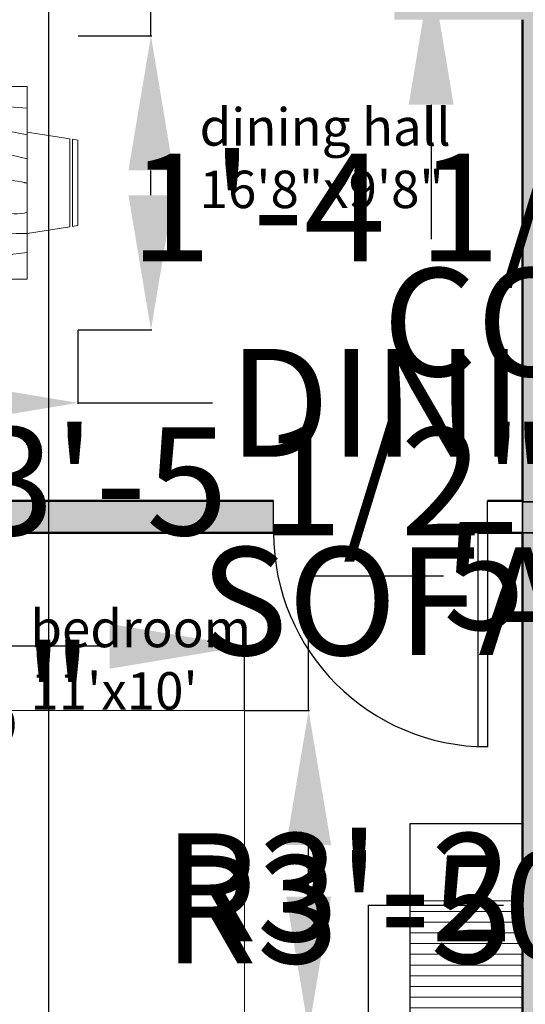
# Model space of a CAD drawing. Units: inches. Extents: x 25 to 82118, y 10 to 6494.
# Tile 4 of 9: x 40833 to 40928, y 3189 to 3373. Entities that reach past the tile are written whole.
import ezdxf

# ---------------------------------------------------------------- set-up
doc = ezdxf.new("R2010")
doc.units = ezdxf.units.IN
doc.header["$MEASUREMENT"] = 0
for name, color, linetype, lineweight in [('A-ANNO-DIMS', 2, 'Continuous', 18), ('A-AREA-IDEN', 7, 'Continuous', 25), ('A-DOOR', 3, 'Continuous', 25), ('A-FLOR-CASE', 8, 'Continuous', 25), ('A-FLOR-CASE-PATT', 9, 'Continuous', 13), ('A-FURN', 8, 'Continuous', 18), ('A-WALL', 7, 'Continuous', 50)]:
    doc.layers.add(name, color=color, linetype=linetype, lineweight=lineweight)
doc.layers.add('A-COLS', color=30, linetype='Continuous', lineweight=35, true_color=0xf26722)
doc.layers.add('A-WALL-PATT', color=18, linetype='Continuous', lineweight=13, true_color=0x000000)
doc.styles.get("Standard").update_dxf_attribs({"font": 'arial.ttf'})
doc.dimstyles.get("Standard").update_dxf_attribs({"dimtxt": 20.18, "dimasz": 25.18, "dimexe": 0.18, "dimexo": 0.0625, "dimgap": 0.09, "dimtad": 0, "dimtih": 1, "dimtoh": 1, "dimdec": 0, "dimzin": 0, "dimdsep": 46, "dimlunit": 3, "dimtxsty": 'Standard', "dimcen": 0.09, "dimadec": 0, "dimazin": 0, "dimtfac": 1, "dimtdec": 0, "dimtofl": 0, "dimtmove": 0, "dimatfit": 3, "dimfxl": 1, "dimtolj": 1, "dimtzin": 0, "dimarcsym": 0})

# ---------------------------------------------------------------- blocks, each defined once
blk = doc.blocks.new('Bed - Queen')
for p, q in [((0, -80.00003), (0, 0)), ((0, 0), (59.99999, 0)), ((59.99999, 0), (59.99999, -80.00003)), ((7.99999, -1.2), (28.79998, -1.2)), ((7.99999, -14.4), (7.99999, -1.2)), ((28.79998, -1.2), (28.79998, -14.4)), ((31.19999, -1.2), (51.99999, -1.2)), ((31.19999, -14.4), (31.19999, -1.2)), ((51.99999, -1.2), (51.99999, -16.4)), ((0, -14.4), (44.8, -14.4)), ((59.99999, -29.6), (44.8, -14.4)), ((44.8, -14.4), (44.8, -29.6)), ((51.99999, -16.4), (46.79936, -16.4)), ((44.8, -16.8), (0, -16.8)), ((44.8, -29.6), (59.99999, -29.6)), ((59.99999, -80.00003), (0, -80.00003))]:
    blk.add_line(p, q)
blk = doc.blocks.new('Dining Set - 36 x 72 in.')
for p, q in [((-22.2343, 26.00059), (-23.4847, 17.99762)), ((-22.2304, 26), (-5.7608, 26)), ((-22, 27.5), (-22.1562, 26.50042)), ((-5.8416, 26.5), (-22.1534, 26.5)), ((-22, 27.5), (-6, 27.5)), ((-5.8437, 26.49966), (-6, 27.5)), ((-4.5152, 17.99762), (-5.7655, 25.99926)), ((5.7657, 26.00059), (4.5153, 17.99762)), ((5.7696, 26), (22.2392, 26)), ((6, 27.5), (5.8438, 26.50042)), ((22.1584, 26.5), (5.8466, 26.5)), ((6, 27.5), (22, 27.5)), ((22.1563, 26.49966), (22, 27.5)), ((23.4848, 17.99762), (22.2345, 25.99926)), ((36, 18), (-36, 18)), ((-36, 18), (-36, -18)), ((36, -18), (36, 18)), ((-44.0006, 8.23428), (-35.9976, 9.48474)), ((44.0006, 8.23428), (35.9976, 9.48474)), ((-45.5, 8), (-44.5004, 8.15617)), ((-45.5, 8), (-45.5, -8)), ((-44.5, -8.15843), (-44.5, 8.15338)), ((-44, 8.23041), (-44, -8.23915)), ((44, 8.23041), (44, -8.23915)), ((44.5, -8.15843), (44.5, 8.15338)), ((45.5, 8), (44.5005, 8.15617)), ((45.5, 8), (45.5, -8)), ((-44.4997, -8.15631), (-45.5, -8)), ((-35.9976, -9.48476), (-43.9993, -8.2345)), ((35.9976, -9.48476), (43.9993, -8.2345)), ((44.4997, -8.15631), (45.5, -8)), ((-36, -18), (36, -18)), ((-22.2343, -26.0006), (-23.4847, -17.99762)), ((-4.5152, -17.99762), (-5.7655, -25.99928)), ((5.7657, -26.0006), (4.5153, -17.99762)), ((23.4848, -17.99762), (22.2345, -25.99928)), ((-22.2304, -26), (-5.7608, -26)), ((-22, -27.5), (-22.1562, -26.50044)), ((-5.8416, -26.5), (-22.1534, -26.5)), ((-22, -27.5), (-6, -27.5)), ((-5.8437, -26.49967), (-6, -27.5)), ((5.7696, -26), (22.2392, -26)), ((6, -27.5), (5.8438, -26.50044)), ((22.1584, -26.5), (5.8466, -26.5)), ((6, -27.5), (22, -27.5)), ((22.1563, -26.49967), (22, -27.5))]:
    blk.add_line(p, q)
for points in [[(-36, 15), (-31.1772, 14.97754), (-26.8079, 14.91406), (-22.8538, 14.81543), (-19.276, 14.6875), (-16.0362, 14.53613), (-13.0957, 14.36718), (-10.4159, 14.18652), (-7.9583, 14), (-5.6904, 13.81315), (-3.6035, 13.63021), (-1.6954, 13.45508), (0.0365, 13.29166), (1.5945, 13.14388), (2.9811, 13.01562), (4.1988, 12.9108), (5.25, 12.83333), (6.1393, 12.78613), (6.8802, 12.76823), (7.4883, 12.77767), (7.9792, 12.8125), (8.3685, 12.87077), (8.6719, 12.95052), (8.9049, 13.0498), (9.0833, 13.16666), (9.2205, 13.29899), (9.3216, 13.44401), (9.3895, 13.59879), (9.4271, 13.76041), (9.4373, 13.92594), (9.4232, 14.09245), (9.3875, 14.257), (9.3333, 14.41666), (9.2638, 14.56917), (9.1836, 14.71484), (9.0975, 14.85465), (9.0104, 14.98958), (8.9272, 15.1206), (8.8529, 15.2487), (8.7922, 15.37483), (8.75, 15.5), (8.7305, 15.62467), (8.7344, 15.74739), (8.7617, 15.86621), (8.8125, 15.97916), (8.8867, 16.08431), (8.9844, 16.17968), (9.1055, 16.26334), (9.25, 16.33333), (9.4189, 16.38802), (9.6172, 16.42708), (9.8506, 16.45052), (10.125, 16.45833), (10.4463, 16.45052), (10.8203, 16.42708), (11.2529, 16.38802), (11.75, 16.33333), (12.3184, 16.26318), (12.9694, 16.17838), (13.7151, 16.07991), (14.5677, 15.96875), (15.5395, 15.84586), (16.6426, 15.71224), (17.8893, 15.56884), (19.2917, 15.41666), (20.859, 15.25667), (22.5879, 15.08984), (24.4721, 14.91715), (26.5052, 14.73958), (28.6809, 14.5581), (30.9929, 14.3737), (33.4347, 14.18733), (36, 14)], [(-36, 10), (-28.9766, 10.14274), (-23.1725, 10.20442), (-18.4241, 10.19775), (-14.5677, 10.13541), (-11.4399, 10.03011), (-8.877, 9.89453), (-6.7154, 9.74137), (-4.7917, 9.58333), (-2.9698, 9.43082), (-1.2246, 9.28515), (0.4415, 9.14534), (2.026, 9.01041), (3.5266, 8.87939), (4.9408, 8.7513), (6.266, 8.62516), (7.5, 8.5), (8.6411, 8.37549), (9.6914, 8.2539), (10.6538, 8.13818), (11.5312, 8.03125), (12.3267, 7.93603), (13.043, 7.85547), (13.6831, 7.79248), (14.25, 7.75), (14.7471, 7.7303), (15.1797, 7.73307), (15.5537, 7.75732), (15.875, 7.80208), (16.1494, 7.86637), (16.3828, 7.94922), (16.5811, 8.04964), (16.75, 8.16666), (16.8944, 8.29915), (17.0143, 8.44531), (17.1089, 8.60319), (17.1771, 8.77083), (17.218, 8.94629), (17.2305, 9.1276), (17.2137, 9.31282), (17.1667, 9.5), (17.0895, 9.6875), (16.987, 9.875), (16.8649, 10.0625), (16.7292, 10.25), (16.5856, 10.4375), (16.4401, 10.625), (16.2985, 10.8125), (16.1667, 11), (16.05, 11.18733), (15.9518, 11.3737), (15.8752, 11.5581), (15.8229, 11.73958), (15.798, 11.91715), (15.8034, 12.08984), (15.842, 12.25667), (15.9167, 12.41666), (16.0295, 12.56836), (16.1784, 12.70833), (16.3605, 12.83268), (16.5729, 12.9375), (16.8127, 13.01888), (17.0768, 13.07291), (17.3625, 13.0957), (17.6667, 13.08333), (17.9894, 13.03312), (18.3418, 12.94726), (18.7382, 12.82918), (19.1927, 12.68229), (19.7195, 12.51001), (20.3327, 12.31575), (21.0465, 12.10294), (21.875, 11.875), (22.8357, 11.63354), (23.959, 11.37304), (25.2786, 11.08618), (26.8282, 10.76562), (28.6414, 10.40405), (30.752, 9.99414), (33.1936, 9.52856), (36, 9)], [(-36, 5.5), (-30.7157, 5.3348), (-26.069, 5.20963), (-21.9946, 5.11767), (-18.4271, 5.05208), (-15.3009, 5.00602), (-12.5508, 4.97265), (-10.1112, 4.94515), (-7.9167, 4.91666), (-5.909, 4.88167), (-4.0586, 4.83984), (-2.3429, 4.79215), (-0.7396, 4.73958), (0.7739, 4.6831), (2.22, 4.6237), (3.6213, 4.56233), (5, 4.5), (6.373, 4.43782), (7.7344, 4.3776), (9.0723, 4.32129), (10.375, 4.27083), (11.6309, 4.22819), (12.8281, 4.19531), (13.9551, 4.17415), (15, 4.16666), (15.954, 4.17448), (16.819, 4.19791), (17.6001, 4.23698), (18.3021, 4.29166), (18.9299, 4.36198), (19.4883, 4.44791), (19.9823, 4.54948), (20.4167, 4.66666), (20.7969, 4.79899), (21.1302, 4.94401), (21.4245, 5.09879), (21.6875, 5.26041), (21.9271, 5.42594), (22.1511, 5.59245), (22.3672, 5.757), (22.5834, 5.91666), (22.8065, 6.06868), (23.0404, 6.21093), (23.2879, 6.34147), (23.5521, 6.45833), (23.8358, 6.55957), (24.142, 6.64323), (24.4735, 6.70735), (24.8334, 6.75), (25.2235, 6.76969), (25.642, 6.76692), (26.0858, 6.74267), (26.5521, 6.69791), (27.0379, 6.63362), (27.5404, 6.55078), (28.0565, 6.45036), (28.5834, 6.33333), (29.1242, 6.19987), (29.7071, 6.04687), (30.3661, 5.87044), (31.1354, 5.66666), (32.0493, 5.43164), (33.142, 5.16146), (34.4475, 4.85221), (36, 4.5)], [(-36, -1), (-30.7915, -0.6591), (-26.0195, -0.38216), (-21.6519, -0.16284), (-17.6563, 0.00521), (-14.0005, 0.12833), (-10.6523, 0.21289), (-7.5796, 0.26522), (-4.75, 0.29166), (-2.134, 0.29793), (0.2878, 0.28711), (2.5317, 0.26163), (4.6146, 0.22396), (6.5529, 0.17651), (8.3633, 0.12174), (10.0623, 0.06209), (11.6667, 0), (13.1899, -0.06201), (14.6341, -0.1211), (15.9982, -0.17432), (17.2813, -0.21875), (18.4823, -0.25147), (19.6003, -0.26953), (20.6343, -0.27002), (21.5834, -0.25), (22.4481, -0.20768), (23.2357, -0.14584), (23.9549, -0.06836), (24.6146, 0.02083), (25.2235, 0.11784), (25.7904, 0.21875), (26.3241, 0.31966), (26.8334, 0.41666), (27.3265, 0.50618), (27.8099, 0.58593), (28.2894, 0.65397), (28.7709, 0.70833), (29.2601, 0.74707), (29.763, 0.76823), (30.2855, 0.76985), (30.8334, 0.75), (31.4088, 0.70784), (31.9994, 0.64713), (32.589, 0.57275), (33.1615, 0.48958), (33.7008, 0.4025), (34.1908, 0.3164), (34.6153, 0.23616), (34.9584, 0.16666), (35.2099, 0.11165), (35.3848, 0.07031), (35.504, 0.04069), (35.5886, 0.02083), (35.6594, 0.00879), (35.7377, 0.0026), (35.8442, 0.00032), (36, 0)], [(-36, -6.5), (-27.1843, -6.31267), (-20.084, -6.1263), (-14.469, -5.9419), (-10.1094, -5.76042), (-6.7752, -5.58285), (-4.2363, -5.41016), (-2.2629, -5.24333), (-0.625, -5.08334), (0.8708, -4.93099), (2.2715, -4.78646), (3.5872, -4.64974), (4.8281, -4.52084), (6.0046, -4.39974), (7.127, -4.28646), (8.2053, -4.18099), (9.25, -4.08334), (10.2705, -3.99382), (11.2734, -3.91407), (12.2647, -3.84603), (13.25, -3.79167), (14.2354, -3.75293), (15.2266, -3.73177), (16.2295, -3.73015), (17.25, -3.75), (18.2912, -3.79248), (19.3451, -3.85547), (20.4009, -3.93604), (21.4479, -4.03125), (22.4754, -4.13819), (23.4727, -4.25391), (24.4289, -4.37549), (25.3334, -4.5), (26.1785, -4.62492), (26.9694, -4.74935), (27.7145, -4.87281), (28.4219, -4.99479), (29.1, -5.11483), (29.7572, -5.23242), (30.4016, -5.34709), (31.0417, -5.45834), (31.6837, -5.56437), (32.3262, -5.65821), (32.9658, -5.73153), (33.599, -5.77604), (34.2224, -5.78345), (34.8327, -5.74545), (35.4264, -5.65373), (36, -5.5)], [(-36, -10), (-26.4022, -9.81299), (-18.4675, -9.62891), (-11.9839, -9.45069), (-6.7396, -9.28125), (-2.5226, -9.12354), (0.8789, -8.98047), (3.6769, -8.85498), (6.0833, -8.75), (8.2767, -8.66765), (10.3021, -8.60677), (12.1712, -8.56543), (13.8958, -8.54167), (15.4876, -8.53353), (16.9583, -8.53907), (18.3197, -8.55632), (19.5834, -8.58334), (20.7616, -8.61841), (21.8685, -8.66081), (22.9188, -8.71004), (23.9271, -8.76563), (24.9081, -8.82707), (25.8763, -8.89388), (26.8465, -8.96558), (27.8334, -9.04167), (28.8474, -9.12118), (29.8828, -9.20117), (30.93, -9.27824), (31.9792, -9.34896), (33.0205, -9.40991), (34.0443, -9.45768), (35.0407, -9.48885), (36, -9.5)], [(-36, -14.5), (-30.0881, -14.33513), (-25.0332, -14.21224), (-20.7312, -14.12647), (-17.0781, -14.07292), (-13.97, -14.04671), (-11.3027, -14.04297), (-8.9724, -14.05681), (-6.875, -14.08334), (-4.9224, -14.11833), (-3.0905, -14.16016), (-1.3709, -14.20785), (0.2448, -14.26042), (1.7647, -14.3169), (3.1973, -14.3763), (4.5507, -14.43767), (5.8333, -14.5), (7.0554, -14.5621), (8.235, -14.62175), (9.3922, -14.67652), (10.5469, -14.72396), (11.7192, -14.76164), (12.929, -14.78711), (14.1965, -14.79794), (15.5417, -14.79167), (16.9933, -14.76424), (18.6152, -14.70508), (20.4804, -14.60197), (22.6615, -14.44271), (25.2312, -14.21509), (28.2624, -13.9069), (31.8277, -13.50594), (36, -13)]]:
    blk.add_lwpolyline(points)
blk = doc.blocks.new('*U12')
for p, q in [((0, 0), (0, -6)), ((40, 0), (40, -6))]:
    blk.add_line(p, q)
blk.add_lwpolyline([(0, 0), (0, 40), (1.75, 40), (1.75, 0)], close=True)
blk.add_arc((0, 0), 40, 0, 90)
blk = doc.blocks.new('POST-INTERIOR-6IN')
h = blk.add_hatch(color=256)
h.dxf.hatch_style = 1
h.paths.add_polyline_path([(6, 5.8), (0, 5.8), (0, 0), (6, 0)])
blk.add_lwpolyline([(6, 5.8), (0, 5.8), (0, 0), (6, 0)], close=True)
blk = doc.blocks.new('*D25')
at = {"layer": 'A-ANNO-DIMS', "color": 0, "lineweight": -2, "transparency": 16777216}
for p, q in [((40724.56, 3429.21), (40724.56, 3454.39)), ((40724.56, 3454.39), (40749.74, 3454.39)), ((40723.27, 3404.03), (40724.74, 3404.03)), ((40723.27, 3395.03), (40724.74, 3395.03)), ((40724.56, 3369.85), (40724.56, 3344.67))]:
    blk.add_line(p, q, dxfattribs=at)
at = {"layer": 'A-ANNO-DIMS', "color": 0, "transparency": 16777216}
for points in [[(40720.36, 3429.21), (40728.76, 3429.21), (40724.56, 3404.03)], [(40720.36, 3369.85), (40728.76, 3369.85), (40724.56, 3395.03)]]:
    blk.add_solid(points, dxfattribs=at)
at = {"layer": 'Defpoints', "color": 0, "transparency": 16777216}
for p in [(40723.21, 3404.03), (40724.56, 3404.03), (40723.21, 3395.03)]:
    blk.add_point(p, dxfattribs=at)
at = {"layer": 'A-ANNO-DIMS', "color": 0, "transparency": 16777216, "insert": (40876.22, 3454.39), "char_height": 20.18, "attachment_point": 5}
blk.add_mtext('\\A1;COLUMN 0\'-9" TYP.', dxfattribs=at)
blk = doc.blocks.new('*D27')
at = {"layer": 'A-ANNO-DIMS', "color": 0, "lineweight": -2, "transparency": 16777216}
for p, q in [((40903.21, 3382.03), (40903.21, 3381.02)), ((40909.21, 3382.03), (40909.21, 3381.02)), ((40878.03, 3381.2), (40852.85, 3381.2)), ((40934.39, 3381.2), (40959.57, 3381.2))]:
    blk.add_line(p, q, dxfattribs=at)
at = {"layer": 'A-ANNO-DIMS', "color": 0, "transparency": 16777216}
for points in [[(40878.03, 3385.39), (40878.03, 3377), (40903.21, 3381.2)], [(40934.39, 3385.39), (40934.39, 3377), (40909.21, 3381.2)]]:
    blk.add_solid(points, dxfattribs=at)
at = {"layer": 'Defpoints', "color": 0, "transparency": 16777216}
for p in [(40903.21, 3382.1), (40909.21, 3382.1), (40909.21, 3381.2)]:
    blk.add_point(p, dxfattribs=at)
at = {"layer": 'A-ANNO-DIMS', "color": 0, "transparency": 16777216, "insert": (41062.95, 3381.2), "char_height": 20.18, "attachment_point": 5}
blk.add_mtext('\\A1;POST 0\'-6" TYP.', dxfattribs=at)
blk = doc.blocks.new('*D28')
at = {"layer": 'A-ANNO-DIMS', "color": 0, "lineweight": -2, "transparency": 16777216}
for p, q in [((40910.11, 3413.07), (40910.11, 3438.25)), ((40910.11, 3438.25), (40935.29, 3438.25)), ((40909.27, 3387.89), (40910.29, 3387.89)), ((40909.27, 3382.1), (40910.29, 3382.1)), ((40910.11, 3356.92), (40910.11, 3331.74))]:
    blk.add_line(p, q, dxfattribs=at)
at = {"layer": 'A-ANNO-DIMS', "color": 0, "transparency": 16777216}
for points in [[(40905.91, 3413.07), (40914.31, 3413.07), (40910.11, 3387.89)], [(40905.91, 3356.92), (40914.31, 3356.92), (40910.11, 3382.1)]]:
    blk.add_solid(points, dxfattribs=at)
at = {"layer": 'Defpoints', "color": 0, "transparency": 16777216}
for p in [(40909.21, 3387.89), (40910.11, 3387.89), (40909.21, 3382.1)]:
    blk.add_point(p, dxfattribs=at)
at = {"layer": 'A-ANNO-DIMS', "color": 0, "transparency": 16777216, "insert": (40996.88, 3438.25), "char_height": 20.18, "attachment_point": 5}
blk.add_mtext('\\A1;0\'-6" TYP.', dxfattribs=at)
blk = doc.blocks.new('*D32')
at = {"layer": 'A-ANNO-DIMS', "color": 0, "lineweight": -2, "transparency": 16777216}
for p, q in [((40898.43, 3182), (40898.43, 3207.18)), ((40898.43, 3207.18), (40923.61, 3207.18)), ((40890.7, 3156.82), (40898.61, 3156.82)), ((40890.7, 3147.82), (40898.61, 3147.82)), ((40898.43, 3122.64), (40898.43, 3097.46))]:
    blk.add_line(p, q, dxfattribs=at)
at = {"layer": 'A-ANNO-DIMS', "color": 0, "transparency": 16777216}
for points in [[(40894.24, 3182), (40902.63, 3182), (40898.43, 3156.82)], [(40894.24, 3122.64), (40902.63, 3122.64), (40898.43, 3147.82)]]:
    blk.add_solid(points, dxfattribs=at)
at = {"layer": 'Defpoints', "color": 0, "transparency": 16777216}
for p in [(40890.63, 3156.82), (40898.43, 3156.82), (40890.63, 3147.82)]:
    blk.add_point(p, dxfattribs=at)
at = {"layer": 'A-ANNO-DIMS', "color": 0, "transparency": 16777216, "insert": (40985.21, 3207.18), "char_height": 20.18, "attachment_point": 5}
blk.add_mtext('\\A1;0\'-9" TYP.', dxfattribs=at)
blk = doc.blocks.new('*D35')
at = {"layer": 'A-ANNO-DIMS', "color": 0, "lineweight": -2, "transparency": 16777216}
for p, q in [((40795.21, 3255.62), (40770.03, 3255.62)), ((40795.21, 3243.68), (40795.21, 3255.8)), ((40850.03, 3255.62), (40820.39, 3255.62)), ((40875.21, 3243.68), (40875.21, 3255.8))]:
    blk.add_line(p, q, dxfattribs=at)
at = {"layer": 'A-ANNO-DIMS', "color": 0, "transparency": 16777216}
for points in [[(40820.39, 3259.82), (40820.39, 3251.42), (40795.21, 3255.62)], [(40850.03, 3259.82), (40850.03, 3251.42), (40875.21, 3255.62)]]:
    blk.add_solid(points, dxfattribs=at)
at = {"layer": 'Defpoints', "color": 0, "transparency": 16777216}
for p in [(40795.21, 3255.62), (40795.21, 3243.62), (40875.21, 3243.62)]:
    blk.add_point(p, dxfattribs=at)
at = {"layer": 'A-ANNO-DIMS', "color": 0, "transparency": 16777216, "insert": (40621.51, 3255.62), "char_height": 20.18, "attachment_point": 5}
blk.add_mtext('\\A1;QUEEN BED 6\'-8" TYP.', dxfattribs=at)
blk = doc.blocks.new('*D36')
at = {"layer": 'A-ANNO-DIMS', "color": 0, "lineweight": -2, "transparency": 16777216}
for p, q in [((40887.21, 3243.62), (40887.21, 3268.8)), ((40887.21, 3268.8), (40912.39, 3268.8)), ((40875.27, 3243.62), (40887.39, 3243.62)), ((40887.21, 3208.8), (40887.21, 3218.44)), ((40875.27, 3183.62), (40887.39, 3183.62))]:
    blk.add_line(p, q, dxfattribs=at)
at = {"layer": 'A-ANNO-DIMS', "color": 0, "transparency": 16777216}
for points in [[(40883.01, 3218.44), (40891.41, 3218.44), (40887.21, 3243.62)], [(40883.01, 3208.8), (40891.41, 3208.8), (40887.21, 3183.62)]]:
    blk.add_solid(points, dxfattribs=at)
at = {"layer": 'Defpoints', "color": 0, "transparency": 16777216}
for p in [(40875.21, 3243.62), (40887.21, 3243.62), (40875.21, 3183.62)]:
    blk.add_point(p, dxfattribs=at)
at = {"layer": 'A-ANNO-DIMS', "color": 0, "transparency": 16777216, "insert": (40973.98, 3268.8), "char_height": 20.18, "attachment_point": 5}
blk.add_mtext('\\A1;5\'-0" TYP.', dxfattribs=at)
blk = doc.blocks.new('*D42')
at = {"layer": 'A-ANNO-DIMS', "color": 0, "lineweight": -2, "transparency": 16777216}
for p, q in [((40725.21, 3248.99), (40725.21, 3245.52)), ((40740.15, 3248.99), (40740.15, 3245.52)), ((40700.03, 3245.7), (40674.85, 3245.7)), ((40765.33, 3245.7), (40790.51, 3245.7))]:
    blk.add_line(p, q, dxfattribs=at)
at = {"layer": 'A-ANNO-DIMS', "color": 0, "transparency": 16777216}
for points in [[(40700.03, 3249.89), (40700.03, 3241.5), (40725.21, 3245.7)], [(40765.33, 3249.89), (40765.33, 3241.5), (40740.15, 3245.7)]]:
    blk.add_solid(points, dxfattribs=at)
at = {"layer": 'Defpoints', "color": 0, "transparency": 16777216}
for p in [(40725.21, 3249.06), (40740.15, 3249.06), (40740.15, 3245.7)]:
    blk.add_point(p, dxfattribs=at)
at = {"layer": 'A-ANNO-DIMS', "color": 0, "transparency": 16777216, "insert": (40816.47, 3245.7), "char_height": 20.18, "attachment_point": 5}
blk.add_mtext('\\A1;1\'-3"', dxfattribs=at)
blk = doc.blocks.new('*D43')
at = {"layer": 'A-ANNO-DIMS', "color": 0, "lineweight": -2, "transparency": 16777216}
for p, q in [((41029.25, 3357.91), (41029.25, 3383.09)), ((41024.37, 3332.73), (41029.43, 3332.73)), ((41024.37, 3299.75), (41029.43, 3299.75)), ((41029.25, 3274.57), (41029.25, 3249.39))]:
    blk.add_line(p, q, dxfattribs=at)
at = {"layer": 'A-ANNO-DIMS', "color": 0, "transparency": 16777216}
for points in [[(41025.05, 3357.91), (41033.45, 3357.91), (41029.25, 3332.73)], [(41025.05, 3274.57), (41033.45, 3274.57), (41029.25, 3299.75)]]:
    blk.add_solid(points, dxfattribs=at)
at = {"layer": 'Defpoints', "color": 0, "transparency": 16777216}
for p in [(41024.3, 3332.73), (41029.25, 3332.73), (41024.3, 3299.75)]:
    blk.add_point(p, dxfattribs=at)
at = {"layer": 'A-ANNO-DIMS', "color": 0, "transparency": 16777216, "insert": (41029.25, 3316.24), "char_height": 20.18, "attachment_point": 5}
blk.add_mtext('\\A1;COFFEE TABLE 2\'-9"', dxfattribs=at)
blk = doc.blocks.new('*D44')
at = {"layer": 'A-ANNO-DIMS', "color": 0, "lineweight": -2, "transparency": 16777216}
for p, q in [((40982.63, 3337.68), (40957.45, 3337.68)), ((41007.81, 3332.8), (41007.81, 3337.86)), ((41024.3, 3332.8), (41024.3, 3337.86)), ((41049.48, 3337.68), (41074.66, 3337.68))]:
    blk.add_line(p, q, dxfattribs=at)
at = {"layer": 'A-ANNO-DIMS', "color": 0, "transparency": 16777216}
for points in [[(40982.63, 3341.88), (40982.63, 3333.48), (41007.81, 3337.68)], [(41049.48, 3341.88), (41049.48, 3333.48), (41024.3, 3337.68)]]:
    blk.add_solid(points, dxfattribs=at)
at = {"layer": 'Defpoints', "color": 0, "transparency": 16777216}
for p in [(41007.81, 3337.68), (41007.81, 3332.73), (41024.3, 3332.73)]:
    blk.add_point(p, dxfattribs=at)
at = {"layer": 'A-ANNO-DIMS', "color": 0, "transparency": 16777216, "insert": (40907.98, 3337.68), "char_height": 20.18, "attachment_point": 5}
blk.add_mtext('\\A1;1\'-4 1/2"', dxfattribs=at)
blk = doc.blocks.new('*D45')
at = {"layer": 'A-ANNO-DIMS', "color": 0, "lineweight": -2, "transparency": 16777216}
for p, q in [((41037.46, 3345.25), (41028.94, 3345.25)), ((41029.12, 3320.07), (41029.12, 3314.42)), ((41037.46, 3289.24), (41028.94, 3289.24)), ((41029.12, 3289.24), (41029.12, 3264.06)), ((41029.12, 3264.06), (41003.94, 3264.06))]:
    blk.add_line(p, q, dxfattribs=at)
at = {"layer": 'A-ANNO-DIMS', "color": 0, "transparency": 16777216}
for points in [[(41024.92, 3320.07), (41033.32, 3320.07), (41029.12, 3345.25)], [(41024.92, 3314.42), (41033.32, 3314.42), (41029.12, 3289.24)]]:
    blk.add_solid(points, dxfattribs=at)
at = {"layer": 'Defpoints', "color": 0, "transparency": 16777216}
for p in [(41037.52, 3345.25), (41029.12, 3289.24), (41037.52, 3289.24)]:
    blk.add_point(p, dxfattribs=at)
at = {"layer": 'A-ANNO-DIMS', "color": 0, "transparency": 16777216, "insert": (40934.78, 3264.06), "char_height": 20.18, "attachment_point": 5}
blk.add_mtext('\\A1;SOFA 4\'-8"', dxfattribs=at)
blk = doc.blocks.new('*D47')
at = {"layer": 'A-ANNO-DIMS', "color": 0, "lineweight": -2, "transparency": 16777216}
for p, q in [((40753.09, 3314.74), (40753.09, 3300.97)), ((40844.09, 3314.74), (40844.09, 3300.97)), ((40778.27, 3301.15), (40818.91, 3301.15)), ((40844.09, 3301.15), (40869.27, 3301.15))]:
    blk.add_line(p, q, dxfattribs=at)
at = {"layer": 'A-ANNO-DIMS', "color": 0, "transparency": 16777216}
for points in [[(40778.27, 3305.35), (40778.27, 3296.95), (40753.09, 3301.15)], [(40818.91, 3305.35), (40818.91, 3296.95), (40844.09, 3301.15)]]:
    blk.add_solid(points, dxfattribs=at)
at = {"layer": 'Defpoints', "color": 0, "transparency": 16777216}
for p in [(40753.09, 3314.8), (40844.09, 3314.8), (40844.09, 3301.15)]:
    blk.add_point(p, dxfattribs=at)
at = {"layer": 'A-ANNO-DIMS', "color": 0, "transparency": 16777216, "insert": (40980.26, 3301.15), "char_height": 20.18, "attachment_point": 5}
blk.add_mtext('\\A1;DINING SET 7\'-7"', dxfattribs=at)
blk = doc.blocks.new('*D48')
at = {"layer": 'A-ANNO-DIMS', "color": 0, "lineweight": -2, "transparency": 16777216}
for p, q in [((40857.74, 3369.8), (40857.74, 3394.98)), ((40857.74, 3394.98), (40882.92, 3394.98)), ((40844.15, 3369.8), (40857.92, 3369.8)), ((40857.74, 3339.98), (40857.74, 3344.62)), ((40844.15, 3314.8), (40857.92, 3314.8))]:
    blk.add_line(p, q, dxfattribs=at)
at = {"layer": 'A-ANNO-DIMS', "color": 0, "transparency": 16777216}
for points in [[(40853.54, 3344.62), (40861.93, 3344.62), (40857.74, 3369.8)], [(40853.54, 3339.98), (40861.93, 3339.98), (40857.74, 3314.8)]]:
    blk.add_solid(points, dxfattribs=at)
at = {"layer": 'Defpoints', "color": 0, "transparency": 16777216}
for p in [(40844.09, 3369.8), (40857.74, 3369.8), (40844.09, 3314.8)]:
    blk.add_point(p, dxfattribs=at)
at = {"layer": 'A-ANNO-DIMS', "color": 0, "transparency": 16777216, "insert": (40910.23, 3394.98), "char_height": 20.18, "attachment_point": 5}
blk.add_mtext('\\A1;4\'-7"', dxfattribs=at)
blk = doc.blocks.new('*D49')
at = {"layer": 'A-ANNO-DIMS', "color": 0, "lineweight": -2, "transparency": 16777216}
for p, q in [((40962.31, 3286.49), (40937.13, 3286.49)), ((40987.49, 3280.33), (40987.49, 3286.67)), ((41028.96, 3280.33), (41028.96, 3286.67)), ((41054.14, 3286.49), (41079.32, 3286.49))]:
    blk.add_line(p, q, dxfattribs=at)
at = {"layer": 'A-ANNO-DIMS', "color": 0, "transparency": 16777216}
for points in [[(40962.31, 3290.68), (40962.31, 3282.29), (40987.49, 3286.49)], [(41054.14, 3290.68), (41054.14, 3282.29), (41028.96, 3286.49)]]:
    blk.add_solid(points, dxfattribs=at)
at = {"layer": 'Defpoints', "color": 0, "transparency": 16777216}
for p in [(40987.49, 3286.49), (40987.49, 3280.26), (41028.96, 3280.26)]:
    blk.add_point(p, dxfattribs=at)
at = {"layer": 'A-ANNO-DIMS', "color": 0, "transparency": 16777216, "insert": (40808.81, 3286.49), "char_height": 20.18, "attachment_point": 5}
blk.add_mtext('\\A1;LOVESEAT 3\'-5 1/2"', dxfattribs=at)
blk = doc.blocks.new('*D51')
at = {"layer": 'A-ANNO-DIMS', "color": 0, "lineweight": -2, "transparency": 16777216}
for p, q in [((40750.31, 3454.92), (40750.31, 3480.1)), ((40746.92, 3429.74), (40750.49, 3429.74)), ((40746.92, 3406.76), (40750.49, 3406.76)), ((40750.31, 3381.58), (40750.31, 3356.4))]:
    blk.add_line(p, q, dxfattribs=at)
at = {"layer": 'A-ANNO-DIMS', "color": 0, "transparency": 16777216}
for points in [[(40746.11, 3454.92), (40754.5, 3454.92), (40750.31, 3429.74)], [(40746.11, 3381.58), (40754.5, 3381.58), (40750.31, 3406.76)]]:
    blk.add_solid(points, dxfattribs=at)
at = {"layer": 'Defpoints', "color": 0, "transparency": 16777216}
for p in [(40746.86, 3429.74), (40750.31, 3429.74), (40746.86, 3406.76)]:
    blk.add_point(p, dxfattribs=at)
at = {"layer": 'A-ANNO-DIMS', "color": 0, "transparency": 16777216, "insert": (40750.31, 3418.25), "char_height": 20.18, "attachment_point": 5}
blk.add_mtext('\\A1;FRIDGE 1\'-11"', dxfattribs=at)
blk = doc.blocks.new('*D55')
at = {"layer": 'A-ANNO-DIMS', "color": 0, "lineweight": -2, "transparency": 16777216}
for p, q in [((40937.89, 3240.76), (40937.89, 3119.41)), ((40977.89, 3240.76), (40977.89, 3119.41)), ((40912.71, 3119.59), (40887.53, 3119.59)), ((41003.07, 3119.59), (41028.25, 3119.59))]:
    blk.add_line(p, q, dxfattribs=at)
at = {"layer": 'A-ANNO-DIMS', "color": 0, "transparency": 16777216}
for points in [[(40912.71, 3123.78), (40912.71, 3115.39), (40937.89, 3119.59)], [(41003.07, 3123.78), (41003.07, 3115.39), (40977.89, 3119.59)]]:
    blk.add_solid(points, dxfattribs=at)
at = {"layer": 'Defpoints', "color": 0, "transparency": 16777216}
for p in [(40937.89, 3240.82), (40977.89, 3240.82), (40977.89, 3119.59)]:
    blk.add_point(p, dxfattribs=at)
at = {"layer": 'A-ANNO-DIMS', "color": 0, "transparency": 16777216, "insert": (41055.16, 3119.59), "char_height": 20.18, "attachment_point": 5}
blk.add_mtext('\\A1;3\'-4"', dxfattribs=at)
blk = doc.blocks.new('*D56')
at = {"layer": 'A-ANNO-DIMS', "color": 0, "lineweight": -2, "transparency": 16777216}
for p, q in [((40778.43, 3531.76), (40778.43, 3119.41)), ((40818.43, 3531.76), (40818.43, 3119.41)), ((40753.25, 3119.59), (40728.07, 3119.59)), ((40843.61, 3119.59), (40868.79, 3119.59))]:
    blk.add_line(p, q, dxfattribs=at)
at = {"layer": 'A-ANNO-DIMS', "color": 0, "transparency": 16777216}
for points in [[(40753.25, 3123.78), (40753.25, 3115.39), (40778.43, 3119.59)], [(40843.61, 3123.78), (40843.61, 3115.39), (40818.43, 3119.59)]]:
    blk.add_solid(points, dxfattribs=at)
at = {"layer": 'Defpoints', "color": 0, "transparency": 16777216}
for p in [(40778.43, 3531.82), (40818.43, 3531.82), (40818.43, 3119.59)]:
    blk.add_point(p, dxfattribs=at)
at = {"layer": 'A-ANNO-DIMS', "color": 0, "transparency": 16777216, "insert": (40895.69, 3119.59), "char_height": 20.18, "attachment_point": 5}
blk.add_mtext('\\A1;3\'-4"', dxfattribs=at)
blk = doc.blocks.new('*D58')
at = {"layer": 'A-ANNO-DIMS', "color": 0, "lineweight": -2, "transparency": 16777216}
for p, q in [((40760.71, 3246.88), (40760.71, 3573.03)), ((40782.73, 3246.88), (40782.73, 3573.03)), ((40735.53, 3572.85), (40710.35, 3572.85)), ((40807.91, 3572.85), (40833.09, 3572.85))]:
    blk.add_line(p, q, dxfattribs=at)
at = {"layer": 'A-ANNO-DIMS', "color": 0, "transparency": 16777216}
for points in [[(40735.53, 3577.05), (40735.53, 3568.66), (40760.71, 3572.85)], [(40807.91, 3577.05), (40807.91, 3568.66), (40782.73, 3572.85)]]:
    blk.add_solid(points, dxfattribs=at)
at = {"layer": 'Defpoints', "color": 0, "transparency": 16777216}
for p in [(40782.73, 3572.85), (40760.71, 3246.82), (40782.73, 3246.82)]:
    blk.add_point(p, dxfattribs=at)
at = {"layer": 'A-ANNO-DIMS', "color": 0, "transparency": 16777216, "insert": (40866.89, 3572.85), "char_height": 20.18, "attachment_point": 5}
blk.add_mtext('\\A1;1\'-10"', dxfattribs=at)
blk = doc.blocks.new('*D67')
at = {"layer": 'A-ANNO-DIMS', "color": 0, "lineweight": -2, "transparency": 16777216}
for p, q in [((40795.21, 3156.88), (40795.21, 3573.03)), ((40838.63, 3156.88), (40838.63, 3573.03)), ((40770.03, 3572.85), (40744.85, 3572.85)), ((40863.81, 3572.85), (40888.99, 3572.85))]:
    blk.add_line(p, q, dxfattribs=at)
at = {"layer": 'A-ANNO-DIMS', "color": 0, "transparency": 16777216}
for points in [[(40770.03, 3577.05), (40770.03, 3568.66), (40795.21, 3572.85)], [(40863.81, 3577.05), (40863.81, 3568.66), (40838.63, 3572.85)]]:
    blk.add_solid(points, dxfattribs=at)
at = {"layer": 'Defpoints', "color": 0, "transparency": 16777216}
for p in [(40838.63, 3572.85), (40795.21, 3156.82), (40838.63, 3156.82)]:
    blk.add_point(p, dxfattribs=at)
at = {"layer": 'A-ANNO-DIMS', "color": 0, "transparency": 16777216, "insert": (40939.41, 3572.85), "char_height": 20.18, "attachment_point": 5}
blk.add_mtext('\\A1;3\'-7 1/2"', dxfattribs=at)
blk = doc.blocks.new('*D71')
at = {"layer": 'A-ANNO-DIMS', "color": 0, "lineweight": -2, "transparency": 16777216}
for p, q in [((41008.23, 3298.32), (41008.23, 3298.5)), ((41008.14, 3298.41), (41008.32, 3298.41)), ((41008.23, 3206.4), (41008.23, 3231.58)), ((40983.05, 3206.4), (41008.23, 3206.4))]:
    blk.add_line(p, q, dxfattribs=at)
at = {"layer": 'A-ANNO-DIMS', "color": 0, "transparency": 16777216}
blk.add_solid([(41004.03, 3231.58), (41012.42, 3231.58), (41008.23, 3256.76)], dxfattribs=at)
at = {"layer": 'Defpoints', "color": 0, "transparency": 16777216}
for p in [(41008.23, 3298.41), (41008.23, 3256.76)]:
    blk.add_point(p, dxfattribs=at)
at = {"layer": 'A-ANNO-DIMS', "color": 0, "transparency": 16777216, "insert": (40922.97, 3206.4), "char_height": 20.18, "attachment_point": 5}
blk.add_mtext('\\A1;R3\'-5 1/2"', dxfattribs=at)
blk = doc.blocks.new('*D72')
at = {"layer": 'A-ANNO-DIMS', "color": 0, "lineweight": -2, "transparency": 16777216}
for p, q in [((41008.14, 3299.19), (41008.32, 3299.19)), ((41008.23, 3299.1), (41008.23, 3299.28)), ((41008.23, 3210.55), (41008.23, 3235.73)), ((40983.05, 3210.55), (41008.23, 3210.55))]:
    blk.add_line(p, q, dxfattribs=at)
at = {"layer": 'A-ANNO-DIMS', "color": 0, "transparency": 16777216}
blk.add_solid([(41004.03, 3235.73), (41012.42, 3235.73), (41008.23, 3260.91)], dxfattribs=at)
at = {"layer": 'Defpoints', "color": 0, "transparency": 16777216}
for p in [(41008.23, 3299.19), (41008.23, 3260.91)]:
    blk.add_point(p, dxfattribs=at)
at = {"layer": 'A-ANNO-DIMS', "color": 0, "transparency": 16777216, "insert": (40922.97, 3210.55), "char_height": 20.18, "attachment_point": 5}
blk.add_mtext('\\A1;R3\'-2 1/2"', dxfattribs=at)

msp = doc.modelspace()

# ---------------------------------------------------------------- hatches: boundary and pattern name
at = {"layer": 'A-FLOR-CASE-PATT'}
h = msp.add_hatch(dxfattribs=at)
h.set_pattern_fill('ANSI31', color=256, scale=16, angle=-45, style=0)
h.paths.add_polyline_path([(40906.2, 3157.44), (40927.21, 3157.44), (40927.21, 3209.44), (40906.2, 3209.44)])
at = {"layer": 'A-WALL-PATT'}
h = msp.add_hatch(color=256, dxfattribs=at)
h.dxf.hatch_style = 1
h.paths.add_polyline_path([(40778.43, 3531.82), (40723.21, 3531.82), (40723.21, 3522.82), (40778.54, 3522.82, -0.01877), (40778.43, 3525.82)])
h.paths.add_polyline_path([(40723.21, 3522.82), (40714.21, 3522.82), (40714.21, 3500.82), (40723.21, 3500.82)])
h.paths.add_polyline_path([(40723.21, 3424.82), (40714.21, 3424.82), (40714.21, 3404.03), (40723.21, 3404.03)])
h.paths.add_polyline_path([(40723.21, 3395.03), (40714.21, 3395.03), (40714.21, 3386.82), (40723.21, 3386.82)])
h.paths.add_polyline_path([(40901.65, 3531.82), (40834.16, 3531.82), (40834.16, 3522.82), (40901.65, 3522.82)])
h.paths.add_polyline_path([(40825.16, 3531.82), (40818.43, 3531.82), (40818.43, 3525.82), (40818.43, 3522.82), (40825.16, 3522.82)])
h.paths.add_polyline_path([(40961.21, 3531.82), (40910.65, 3531.82), (40910.65, 3522.82), (40961.21, 3522.82)])
h.paths.add_polyline_path([(41065.21, 3531.82), (41013.21, 3531.82), (41013.21, 3522.82), (41065.21, 3522.82)])
h.paths.add_polyline_path([(41074.21, 3522.82), (41065.21, 3522.82), (41065.21, 3506.52), (41074.21, 3506.52)])
h.paths.add_polyline_path([(41074.21, 3430.52), (41065.21, 3430.52), (41065.21, 3428.74), (41065.21, 3380.62), (41074.21, 3380.62)])
h.paths.add_polyline_path([(41074.21, 3371.62), (41065.21, 3371.62), (41065.21, 3355.41), (41074.21, 3355.41)])
h.paths.add_polyline_path([(41065.36, 3378.82), (40909.21, 3378.82), (40909.21, 3382.1), (40903.21, 3382.1), (40903.21, 3372.82), (41065.36, 3372.82)])
h.paths.add_polyline_path([(40933.21, 3372.82), (40927.21, 3372.82), (40927.21, 3282.62), (40933.21, 3282.62)])
h.paths.add_polyline_path([(41074.21, 3279.41), (41065.21, 3279.41), (41065.21, 3240.82), (41074.21, 3240.82)])
h.paths.add_polyline_path([(41065.21, 3246.82), (41052.05, 3246.82), (41052.05, 3240.82), (41065.21, 3240.82)])
h.paths.add_polyline_path([(40985.75, 3202.89), (41023.1, 3202.89), (41023.1, 3229.01), (40985.75, 3229.01)], flags=9)
h.paths.add_polyline_path([(40960.75, 3302.54), (40998.1, 3302.54), (40998.1, 3328.66), (40960.75, 3328.66)], flags=9)
h = msp.add_hatch(color=256, dxfattribs=at)
h.dxf.hatch_style = 1
h.paths.add_polyline_path([(40723.21, 3274), (40714.21, 3274), (40714.21, 3212.82), (40723.21, 3212.82), (40723.21, 3240.82), (40760.88, 3240.82, -0.030698), (40760.71, 3243.52), (40760.71, 3246.82), (40723.21, 3246.82)])
h.paths.add_polyline_path([(40789.21, 3246.82), (40782.73, 3246.82), (40782.73, 3243.52), (40782.73, 3240.82), (40789.21, 3240.82)])
h.paths.add_polyline_path([(40795.21, 3276.82), (40880.67, 3276.82), (40880.67, 3282.82), (40789.21, 3282.82), (40789.21, 3240.82), (40795.21, 3240.82), (40795.21, 3243.62)])
h.paths.add_polyline_path([(40795.21, 3240.82), (40789.21, 3240.82), (40789.21, 3156.82), (40723.21, 3156.82), (40723.21, 3147.82), (40838.63, 3147.82), (40838.63, 3156.82), (40795.21, 3156.82)])
h.paths.add_polyline_path([(40723.21, 3184.82), (40714.21, 3184.82), (40714.21, 3156.79), (40723.21, 3156.79), (40723.21, 3156.82)])
h.paths.add_polyline_path([(40924.06, 3156.82), (40890.63, 3156.82), (40890.63, 3147.82), (40924.06, 3147.82)])
h.paths.add_polyline_path([(40933.21, 3240.82), (40937.89, 3240.82), (40937.89, 3246.82), (40933.21, 3246.82), (40933.21, 3276.82), (40927.21, 3276.82), (40927.21, 3156.82), (40933.21, 3156.82)])
h.paths.add_polyline_path([(41000.05, 3246.82), (40977.89, 3246.82), (40977.89, 3240.82), (41000.05, 3240.82)])

# ---------------------------------------------------------------- linework, layer by layer
at = {"layer": 'A-FLOR-CASE'}
for p, q in [((40906.2, 3156.82), (40906.2, 3222.44)), ((40906.2, 3222.44), (40927.21, 3222.44))]:
    msp.add_line(p, q, dxfattribs=at)
at = {"layer": 'A-WALL'}
for p, q in [((40927.21, 3372.82), (40927.21, 3282.82)), ((40880.67, 3282.82), (40789.21, 3282.82)), ((40927.21, 3282.82), (40920.67, 3282.82)), ((40880.67, 3276.82), (40795.21, 3276.82)), ((40927.21, 3276.82), (40918.92, 3276.82)), ((40927.21, 3276.82), (40927.21, 3156.82))]:
    msp.add_line(p, q, dxfattribs=at)

# ---------------------------------------------------------------- block references
at = {"layer": 'A-COLS'}
msp.add_blockref('POST-INTERIOR-6IN', (40927.21, 3276.82), dxfattribs=at)
at = {"layer": 'A-DOOR', "rotation": 180}
msp.add_blockref('*U12', (40920.67, 3276.82), dxfattribs=at)
at = {"layer": 'A-FURN'}
msp.add_blockref('Dining Set - 36 x 72 in.', (40798.59, 3342.3), dxfattribs=at)
at = {"layer": 'A-FURN', "rotation": 90}
msp.add_blockref('Bed - Queen', (40795.21, 3183.62), dxfattribs=at)

# ---------------------------------------------------------------- texts
at = {"layer": 'A-AREA-IDEN', "char_height": 7, "attachment_point": 1}
for s, insert in [('dining hall\\P16\'8"x9\'8"', (40866.83, 3356.25)), ("bedroom\\P11'x10'", (40835.21, 3262.44))]:
    msp.add_mtext_dynamic_manual_height_columns(s, width=132.9687, gutter_width=1, heights=[0], dxfattribs=dict(at, insert=insert))

# ---------------------------------------------------------------- dimensions: what is measured, and where the dimension line sits
at = {"layer": 'A-ANNO-DIMS'}
for base, p1, p2, picture, middle in [((40838.63, 3572.85), (40795.21, 3156.82), (40838.63, 3156.82), '*D67', (40939.41, 3572.85)), ((40782.73, 3572.85), (40760.71, 3246.82), (40782.73, 3246.82), '*D58', (40866.89, 3572.85)), ((40818.43, 3119.59), (40778.43, 3531.82), (40818.43, 3531.82), '*D56', (40895.69, 3119.59)), ((40740.15, 3245.7), (40725.21, 3249.06), (40740.15, 3249.06), '*D42', (40816.47, 3245.7)), ((40977.89, 3119.59), (40937.89, 3240.82), (40977.89, 3240.82), '*D55', (41055.16, 3119.59))]:
    dim = msp.add_linear_dim(base=base, p1=p1, p2=p2, dimstyle='Standard', override={"dimdec": 1, "dimlfac": 1, "dimrnd": 0, "dimzin": 1, "dimdsep": 46, "dimlunit": 4, "dimfrac": 2}, dxfattribs=at)
    dim.commit()
    dim.dimension.update_dxf_attribs({"geometry": picture, "text_midpoint": middle})
for base, p1, p2, angle, text, picture, middle in [((40724.56, 3404.03), (40723.21, 3395.03), (40723.21, 3404.03), 90, 'COLUMN <> TYP.', '*D25', (40876.22, 3454.39)), ((40750.31, 3429.74), (40746.86, 3406.76), (40746.86, 3429.74), 90, 'FRIDGE <>', '*D51', (40750.31, 3418.25)), ((40910.11, 3387.89), (40909.21, 3382.1), (40909.21, 3387.89), 90, '<> TYP.', '*D28', (40996.88, 3438.25)), ((41029.25, 3332.73), (41024.3, 3299.75), (41024.3, 3332.73), 90, 'COFFEE TABLE <>', '*D43', (41029.25, 3316.24)), ((41029.12, 3289.24), (41037.52, 3345.25), (41037.52, 3289.24), 270, 'SOFA <>', '*D45', (40934.78, 3264.06)), ((40987.49, 3286.49), (41028.96, 3280.26), (40987.49, 3280.26), 180, 'LOVESEAT <>', '*D49', (40808.81, 3286.49)), ((40795.21, 3255.62), (40875.21, 3243.62), (40795.21, 3243.62), 180, 'QUEEN BED <> TYP.', '*D35', (40621.51, 3255.62)), ((40887.21, 3243.62), (40875.21, 3183.62), (40875.21, 3243.62), 90, '<> TYP.', '*D36', (40973.98, 3268.8)), ((40898.43, 3156.82), (40890.63, 3147.82), (40890.63, 3156.82), 90, '<> TYP.', '*D32', (40985.21, 3207.18))]:
    dim = msp.add_linear_dim(base=base, p1=p1, p2=p2, angle=angle, text=text, dimstyle='Standard', override={"dimdec": 1, "dimlfac": 1, "dimrnd": 0, "dimzin": 1, "dimdsep": 46, "dimlunit": 4, "dimfrac": 2}, dxfattribs=at)
    dim.commit()
    dim.dimension.update_dxf_attribs({"geometry": picture, "text_midpoint": middle})
for base, p1, p2, text, picture, middle in [((40909.21, 3381.2), (40903.21, 3382.1), (40909.21, 3382.1), 'POST <> TYP.', '*D27', (41062.95, 3381.2)), ((40844.09, 3301.15), (40753.09, 3314.8), (40844.09, 3314.8), 'DINING SET <>', '*D47', (40980.26, 3301.15))]:
    dim = msp.add_linear_dim(base=base, p1=p1, p2=p2, text=text, dimstyle='Standard', override={"dimdec": 1, "dimlfac": 1, "dimrnd": 0, "dimzin": 1, "dimdsep": 46, "dimlunit": 4, "dimfrac": 2}, dxfattribs=at)
    dim.commit()
    dim.dimension.update_dxf_attribs({"geometry": picture, "text_midpoint": middle})
for base, p1, p2, angle, picture, middle in [((40857.74, 3369.8), (40844.09, 3314.8), (40844.09, 3369.8), 90, '*D48', (40910.23, 3394.98)), ((41007.81, 3337.68), (41024.3, 3332.73), (41007.81, 3332.73), 180, '*D44', (40907.98, 3337.68))]:
    dim = msp.add_linear_dim(base=base, p1=p1, p2=p2, angle=angle, dimstyle='Standard', override={"dimdec": 1, "dimlfac": 1, "dimrnd": 0, "dimzin": 1, "dimdsep": 46, "dimlunit": 4, "dimfrac": 2}, dxfattribs=at)
    dim.commit()
    dim.dimension.update_dxf_attribs({"geometry": picture, "text_midpoint": middle})
for center, mpoint, picture, middle in [((41008.23, 3299.19), (41008.23, 3260.91), '*D72', (40922.97, 3210.55)), ((41008.2264, 3298.4101), (41008.226, 3256.7602), '*D71', (40922.9662, 3206.4002))]:
    dim = msp.add_radius_dim(center=center, mpoint=mpoint, dimstyle='Standard', override={"dimdec": 1, "dimlfac": 1, "dimrnd": 0, "dimzin": 1, "dimdsep": 46, "dimlunit": 4, "dimfrac": 2}, dxfattribs=at)
    dim.commit()
    dim.dimension.update_dxf_attribs({"geometry": picture, "text_midpoint": middle})

doc.saveas('drawing.dxf')
